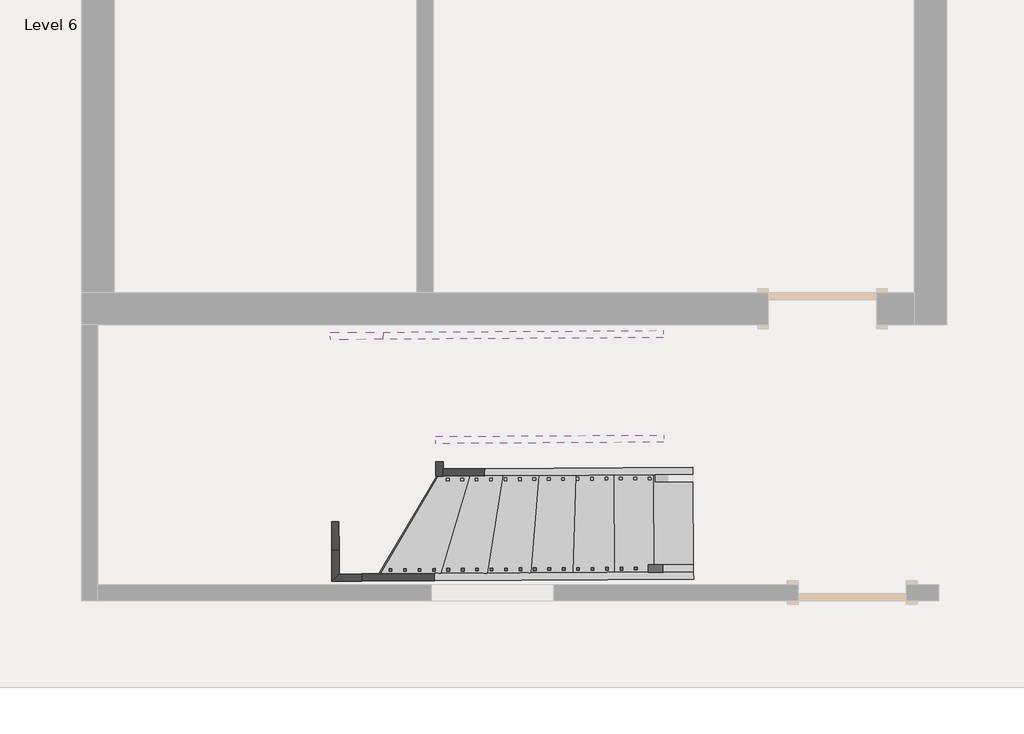
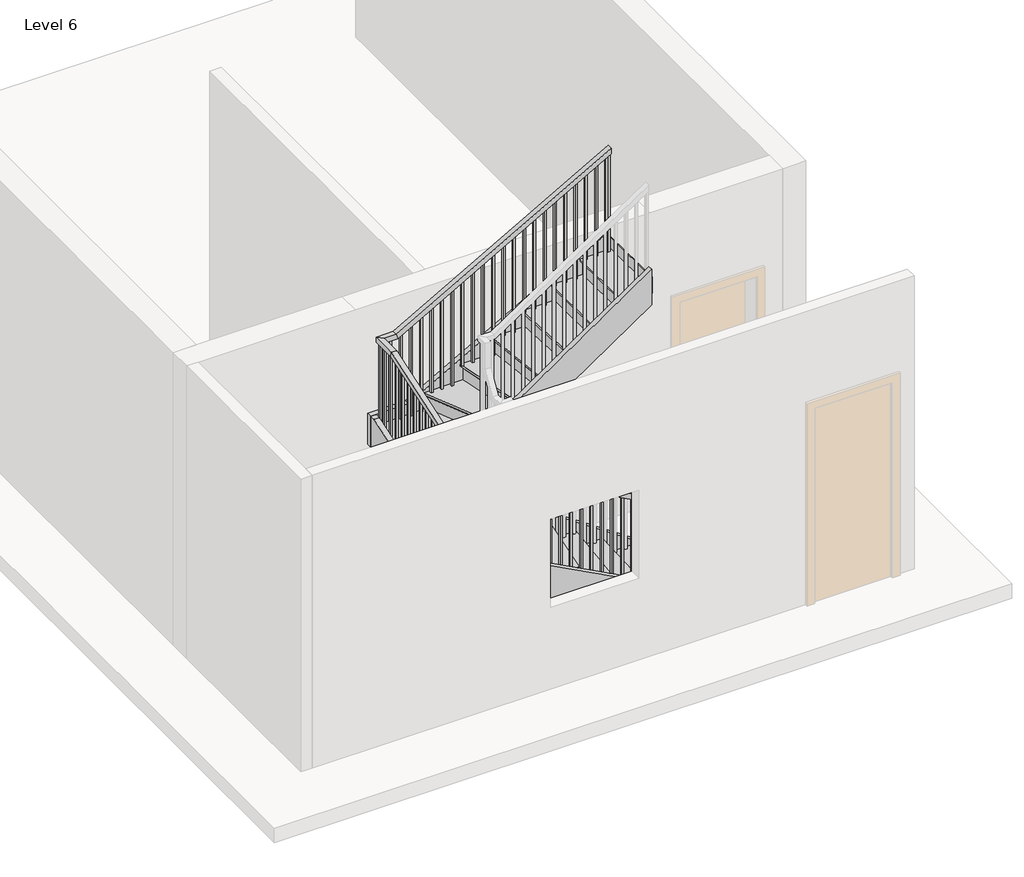
# One storey, part 2 of 2: 9 members, 1 railing, 1 stair flight.
"""IFC4 building model written with IfcOpenShell, lengths in millimetres."""

from ifc_helpers import new_model, si_unit, frame, origin, place, context, project, spatial, polyline, outline, extrude, faceted_brep, transform, mapped, element, save
from components import stair_flight_c1b2dc12

model = new_model("IFC4")

# Units and contexts
model_context = context("Model", 3, world=origin())
ifc_project = project(units=[si_unit("LENGTHUNIT", "METRE", prefix="MILLI")], contexts=[model_context])

# Site, building, storey
site = spatial("IfcSite", under=ifc_project)
building = spatial("IfcBuilding", under=site)
storey = spatial("IfcBuildingStorey", under=building, Name="Level 6", Elevation=12801.6)

# Members
placement = place(None, origin())
element("IfcMember", 1, ObjectType="Stringer - 2\" Width", at=placement, inside=storey, context=model_context, shape_type="SweptSolid", body=[
    extrude(outline(polyline([(-106.4787477, -199.0602913), (0.0, 0.0), (2650.4216713, 0.0), (2487.3820108, -304.8), (91.199922, -304.8), (-106.4787477, -199.0602913)])), frame((-116.1777511, -4276.2080688, 13027.3492487), z_axis=(-0.006129891180436152, 0.9999812120405644, 0.0), x_axis=(-0.881759529662862, -0.005405191516664865, 0.4716682263555568)), (0.0, 0.0, 1.0), 50.8),
])
element("IfcMember", 2, ObjectType="Stringer - 2\" Width", at=placement, inside=storey, context=model_context, shape_type="SweptSolid", body=[
    extrude(outline(polyline([(-2453.5237158, -4239.7350599), (-2453.2123174, -4290.5341055), (-2663.1420684, -4291.8209762), (-2612.6544213, -4240.7105322), (-2453.5237158, -4239.7350599)])), frame((0.0, 0.0, 13931.8029558), z_axis=(0.0, 0.0, 1.0), x_axis=(1.0, 0.0, 0.0)), (0.0, 0.0, 1.0), 345.6659817),
])
element("IfcMember", 3, ObjectType="Stringer - 2\" Width", at=placement, inside=storey, context=model_context, shape_type="SweptSolid", body=[
    extrude(outline(polyline([(-2612.6544213, -4240.7105322), (-2663.1420684, -4291.8209762), (-2664.4731567, -4074.6779247), (-2613.6741111, -4074.3665263), (-2612.6544213, -4240.7105322)])), frame((0.0, 0.0, 13931.8029558), z_axis=(0.0, 0.0, 1.0), x_axis=(1.0, 0.0, 0.0)), (0.0, 0.0, 1.0), 345.6659817),
])
element("IfcMember", 4, ObjectType="Stringer - 2\" Width", at=placement, inside=storey, context=model_context, shape_type="SweptSolid", body=[
    extrude(outline(polyline([(-112.9595567, -326.688092), (0.0, 0.0), (1516.7940002, 1e-07), (1565.1210838, -16.7101466), (1457.9394259, -326.6880919), (-112.9595567, -326.688092)])), frame((-2664.4731567, -4074.6779247, 14277.4689375), z_axis=(0.9999812120405643, 0.006129891180436421, 0.0), x_axis=(-0.005793345483301546, 0.9450798501367781, 0.3267881791215163)), (0.0, 0.0, 1.0), 50.8),
])
element("IfcMember", 5, ObjectType="Stringer - 2\" Width", at=placement, inside=storey, context=model_context, shape_type="SweptSolid", body=[
    extrude(outline(polyline([(-111.800968, -163.7049666), (0.0, 0.0), (2130.8093531, 0.0), (1922.648686, -304.8000001), (94.7979387, -304.8000001), (-111.800968, -163.7049666)])), frame((-120.6930289, -3539.621908, 12999.8391801), z_axis=(-0.006129891180436334, 0.9999812120405643, 0.0), x_axis=(-0.8257797012408892, -0.005062034812924604, 0.5639700885880922)), (0.0, 0.0, 1.0), 50.8),
])
element("IfcMember", 6, ObjectType="Stringer - 2\" Width", at=placement, inside=storey, context=model_context, shape_type="SweptSolid", body=[
    extrude(outline(polyline([(-476.3090819, -288.3824073), (0.0, 0.0), (441.380003, 0.0), (-62.0453256, -304.8), (-466.3690133, -304.8), (-476.3090819, -288.3824073)])), frame((-1931.0711854, -3550.7195376, 14423.9542381), z_axis=(0.9999812120405644, 0.006129891180436035, 0.0), x_axis=(-0.0031747997513555445, 0.5179113315223277, 0.8554284150806007)), (0.0, 0.0, 1.0), 50.8),
])
element("IfcMember", 7, ObjectType="Stringer - 2\" Width", at=placement, inside=storey, context=model_context, shape_type="SweptSolid", body=[
    extrude(outline(polyline([(205.0123517, -304.8), (0.0, 0.0), (1938.1040339, 0.0), (2143.1163855, -304.8), (205.0123517, -304.8)])), frame((-1932.4724786, -3322.1238325, 14468.5006308), z_axis=(-0.006129891180436482, 0.9999812120405644, 0.0), x_axis=(0.8297505463599371, 0.005086376118722323, 0.5581112430271987)), (0.0, 0.0, 1.0), 50.8),
])
element("IfcMember", 8, ObjectType="Stringer - 2\" Width", at=placement, inside=storey, context=model_context, shape_type="SweptSolid", body=[
    extrude(outline(polyline([(-2673.5739172, -2590.0529496), (-2673.8853157, -2539.253904), (-2303.2697085, -2536.982028), (-2302.9583101, -2587.7810735), (-2673.5739172, -2590.0529496)])), frame((0.0, 0.0, 14450.6329153), z_axis=(0.0, 0.0, 1.0), x_axis=(1.0, 0.0, 0.0)), (0.0, 0.0, 1.0), 322.5063717),
])
element("IfcMember", 9, ObjectType="Stringer - 2\" Width", at=placement, inside=storey, context=model_context, shape_type="SweptSolid", body=[
    extrude(outline(polyline([(155.3220552, -282.6400873), (0.0, 0.0), (2252.6037587, 1e-07), (2407.9258139, -282.6400872), (155.3220552, -282.6400873)])), frame((-2302.9583101, -2587.7810735, 14450.6329153), z_axis=(-0.006129891180436272, 0.9999812120405644, 0.0), x_axis=(0.8763695910030255, 0.005372151158450034, 0.4816092606637882)), (0.0, 0.0, 1.0), 50.8),
])

# Railing
element("IfcRailing", 10, ObjectType="Handrail - Rectangular", at=placement, inside=storey, context=model_context, shape_type="SolidModel", body=[
    faceted_brep([(-116.4891496, -4225.4090232, 13885.3333333), (-116.4891496, -4225.4090232, 13827.5022634), (-116.800548, -4174.6099776, 13827.5022634), (-116.800548, -4174.6099776, 13885.3333333), (-2474.2717021, -4239.8622452, 15168.0653479), (-2487.1954725, -4239.941468, 15117.2653479), (-2487.506871, -4189.1424224, 15117.2653479), (-2474.5831006, -4189.0631997, 15168.0653479), (-2612.6544213, -4240.7105322, 15168.0653479), (-2612.6544213, -4240.7105322, 15117.2653479), (-2562.1667742, -4189.6000881, 15117.2653479), (-2562.1667742, -4189.6000881, 15168.0653479), (-2613.899826, -4037.5452114, 15168.0653479), (-2613.9521428, -4029.010664, 15117.2653479), (-2563.1530973, -4028.6992655, 15117.2653479), (-2563.1007804, -4037.2338129, 15168.0653479), (-2621.180916, -2849.7666717, 15578.7734867), (-2621.2332328, -2841.2321243, 15527.9734867), (-2570.4341872, -2840.9207258, 15527.9734867), (-2570.3818704, -2849.4552732, 15578.7734867), (-2622.7748716, -2589.7415511, 15578.7734867), (-2622.7748716, -2589.7415511, 15527.9734867), (-2571.6644276, -2640.2291982, 15527.9734867), (-2571.6644276, -2640.2291982, 15578.7734867), (-2452.0429693, -2588.6949634, 15578.7734867), (-2438.8245474, -2588.6139344, 15527.9734867), (-2438.513149, -2639.41298, 15527.9734867), (-2451.7315708, -2639.494009, 15578.7734867), (-328.8448754, -2575.6797456, 16764.0), (-328.533477, -2626.4787912, 16764.0), (-328.533477, -2626.4787912, 16705.82112), (-328.8448754, -2575.6797456, 16705.82112)], [[[0, 1, 2, 3]], [[1, 0, 4, 5]], [[2, 1, 5, 6]], [[3, 2, 6, 7]], [[0, 3, 7, 4]], [[5, 4, 8, 9]], [[6, 5, 9, 10]], [[7, 6, 10, 11]], [[4, 7, 11, 8]], [[9, 8, 12, 13]], [[10, 9, 13, 14]], [[11, 10, 14, 15]], [[8, 11, 15, 12]], [[13, 12, 16, 17]], [[14, 13, 17, 18]], [[15, 14, 18, 19]], [[12, 15, 19, 16]], [[17, 16, 20, 21]], [[18, 17, 21, 22]], [[19, 18, 22, 23]], [[16, 19, 23, 20]], [[21, 20, 24, 25]], [[22, 21, 25, 26]], [[23, 22, 26, 27]], [[20, 23, 27, 24]], [[28, 29, 30, 31]], [[25, 24, 28, 31]], [[26, 25, 31, 30]], [[27, 26, 30, 29]], [[24, 27, 29, 28]]]),
    extrude(outline(polyline([(233.9170124, 19.05), (1235.5250403, 19.05), (1235.5250403, 0.0), (223.2829877, 0.0), (233.9170124, 19.05)])), frame((-352.4784362, -2610.7502757, 16915.791707), z_axis=(-0.0061298911804362555, 0.9999812120405644, 0.0), x_axis=(0.0, 0.0, -1.0)), (0.0, 0.0, 1.0), 19.05),
    extrude(outline(polyline([(233.9170123, 19.05), (1178.8102421, 19.05), (1178.8102421, 0.0), (223.2829877, 0.0), (233.9170123, 19.05)])), frame((-454.0765273, -2611.3730726, 16859.0769088), z_axis=(-0.0061298911804362555, 0.9999812120405644, 0.0), x_axis=(0.0, 0.0, -1.0)), (0.0, 0.0, 1.0), 19.05),
    extrude(outline(polyline([(233.9170124, 19.05), (1122.095444, 19.05), (1122.095444, 0.0), (223.2829877, 0.0), (233.9170124, 19.05)])), frame((-555.6746185, -2611.9958696, 16802.3621107), z_axis=(-0.0061298911804362555, 0.9999812120405644, 0.0), x_axis=(0.0, 0.0, -1.0)), (0.0, 0.0, 1.0), 19.05),
    extrude(outline(polyline([(233.9170123, 19.05), (1234.7139792, 19.05), (1234.7139792, 0.0), (223.2829877, 0.0), (233.9170123, 19.05)])), frame((-657.2727096, -2612.6186665, 16745.6473125), z_axis=(-0.0061298911804362555, 0.9999812120405644, 0.0), x_axis=(0.0, 0.0, -1.0)), (0.0, 0.0, 1.0), 19.05),
    extrude(outline(polyline([(233.9170123, 19.05), (1177.999181, 19.05), (1177.999181, 0.0), (223.2829876, 0.0), (233.9170123, 19.05)])), frame((-758.8708008, -2613.2414635, 16688.9325143), z_axis=(-0.0061298911804362555, 0.9999812120405644, 0.0), x_axis=(0.0, 0.0, -1.0)), (0.0, 0.0, 1.0), 19.05),
    extrude(outline(polyline([(233.9170123, 19.05), (1121.2843829, 19.05), (1121.2843829, 0.0), (223.2829877, 0.0), (233.9170123, 19.05)])), frame((-860.4688919, -2613.8642604, 16632.2177162), z_axis=(-0.0061298911804362555, 0.9999812120405644, 0.0), x_axis=(0.0, 0.0, -1.0)), (0.0, 0.0, 1.0), 19.05),
    extrude(outline(polyline([(233.9170123, 19.0499999), (1233.902918, 19.0499999), (1233.902918, 0.0), (223.2829876, 0.0), (233.9170123, 19.0499999)])), frame((-962.0669831, -2614.4870574, 16575.502918), z_axis=(-0.0061298911804362555, 0.9999812120405644, 0.0), x_axis=(0.0, 0.0, -1.0)), (0.0, 0.0, 1.0), 19.05),
    extrude(outline(polyline([(233.9170123, 19.05), (1177.1881199, 19.05), (1177.1881199, 0.0), (223.2829877, 0.0), (233.9170123, 19.05)])), frame((-1063.6650742, -2615.1098543, 16518.7881199), z_axis=(-0.0061298911804362555, 0.9999812120405644, 0.0), x_axis=(0.0, 0.0, -1.0)), (0.0, 0.0, 1.0), 19.05),
    extrude(outline(polyline([(233.9170123, 19.05), (1120.4733217, 19.05), (1120.4733217, 0.0), (223.2829876, 0.0), (233.9170123, 19.05)])), frame((-1165.2631653, -2615.7326513, 16462.0733217), z_axis=(-0.0061298911804362555, 0.9999812120405644, 0.0), x_axis=(0.0, 0.0, -1.0)), (0.0, 0.0, 1.0), 19.05),
    extrude(outline(polyline([(233.9170123, 19.05), (1233.0918569, 19.05), (1233.0918569, 0.0), (223.2829877, 0.0), (233.9170123, 19.05)])), frame((-1266.8612565, -2616.3554482, 16405.3585236), z_axis=(-0.0061298911804362555, 0.9999812120405644, 0.0), x_axis=(0.0, 0.0, -1.0)), (0.0, 0.0, 1.0), 19.05),
    extrude(outline(polyline([(233.9170123, 19.05), (1176.3770587, 19.05), (1176.3770587, 0.0), (223.2829876, 0.0), (233.9170123, 19.05)])), frame((-1368.4593476, -2616.9782451, 16348.6437254), z_axis=(-0.0061298911804362555, 0.9999812120405644, 0.0), x_axis=(0.0, 0.0, -1.0)), (0.0, 0.0, 1.0), 19.05),
    extrude(outline(polyline([(233.9170123, 19.05), (1288.995594, 19.05), (1288.995594, 0.0), (223.2829877, 0.0), (233.9170123, 19.05)])), frame((-1470.0574388, -2617.6010421, 16291.9289273), z_axis=(-0.0061298911804362555, 0.9999812120405644, 0.0), x_axis=(0.0, 0.0, -1.0)), (0.0, 0.0, 1.0), 19.05),
    extrude(outline(polyline([(233.9170123, 19.05), (1232.2807958, 19.05), (1232.2807958, 0.0), (223.2829876, 0.0), (233.9170123, 19.05)])), frame((-1571.6555299, -2618.223839, 16235.2141291), z_axis=(-0.0061298911804362555, 0.9999812120405644, 0.0), x_axis=(0.0, 0.0, -1.0)), (0.0, 0.0, 1.0), 19.05),
    extrude(outline(polyline([(233.9170123, 19.05), (1175.5659977, 19.05), (1175.5659977, 0.0), (223.2829877, 0.0), (233.9170123, 19.05)])), frame((-1673.2536211, -2618.846636, 16178.499331), z_axis=(-0.0061298911804362555, 0.9999812120405644, 0.0), x_axis=(0.0, 0.0, -1.0)), (0.0, 0.0, 1.0), 19.05),
    extrude(outline(polyline([(233.9170123, 19.05), (1118.8511995, 19.05), (1118.8511995, 0.0), (223.2829876, 0.0), (233.9170123, 19.05)])), frame((-1774.8517122, -2619.4694329, 16121.7845328), z_axis=(-0.0061298911804362555, 0.9999812120405644, 0.0), x_axis=(0.0, 0.0, -1.0)), (0.0, 0.0, 1.0), 19.05),
    extrude(outline(polyline([(233.9170123, 19.05), (1231.4697347, 19.05), (1231.4697347, 0.0), (223.2829877, 0.0), (233.9170123, 19.05)])), frame((-1876.4498033, -2620.0922299, 16065.0697347), z_axis=(-0.0061298911804362555, 0.9999812120405644, 0.0), x_axis=(0.0, 0.0, -1.0)), (0.0, 0.0, 1.0), 19.05),
    extrude(outline(polyline([(233.9170123, 19.05), (1174.7549365, 19.05), (1174.7549365, 0.0), (223.2829876, 0.0), (233.9170123, 19.05)])), frame((-1978.0478945, -2620.7150268, 16008.3549365), z_axis=(-0.0061298911804362555, 0.9999812120405644, 0.0), x_axis=(0.0, 0.0, -1.0)), (0.0, 0.0, 1.0), 19.05),
    extrude(outline(polyline([(233.9170124, 19.05), (1118.0401384, 19.05), (1118.0401384, 0.0), (223.2829877, 0.0), (233.9170124, 19.05)])), frame((-2079.6459856, -2621.3378238, 15951.6401384), z_axis=(-0.0061298911804362555, 0.9999812120405644, 0.0), x_axis=(0.0, 0.0, -1.0)), (0.0, 0.0, 1.0), 19.05),
    extrude(outline(polyline([(233.9170123, 19.05), (1230.6586735, 19.05), (1230.6586735, 0.0), (223.2829876, 0.0), (233.9170123, 19.05)])), frame((-2181.2440768, -2621.9606207, 15894.9253402), z_axis=(-0.0061298911804362555, 0.9999812120405644, 0.0), x_axis=(0.0, 0.0, -1.0)), (0.0, 0.0, 1.0), 19.05),
    extrude(outline(polyline([(233.9170124, 19.05), (1173.9438754, 19.05), (1173.9438754, 0.0), (223.2829877, 0.0), (233.9170124, 19.05)])), frame((-2282.8421679, -2622.5834176, 15838.2105421), z_axis=(-0.0061298911804362555, 0.9999812120405644, 0.0), x_axis=(0.0, 0.0, -1.0)), (0.0, 0.0, 1.0), 19.05),
    extrude(outline(polyline([(233.9170123, 19.05), (1117.2290772, 19.05), (1117.2290772, 0.0), (223.2829877, 0.0), (233.9170123, 19.05)])), frame((-2384.4402591, -2623.2062146, 15781.4957439), z_axis=(-0.0061298911804362555, 0.9999812120405644, 0.0), x_axis=(0.0, 0.0, -1.0)), (0.0, 0.0, 1.0), 19.05),
    extrude(outline(polyline([(-2505.2047667, -2604.8961439), (-2486.1551246, -2604.7793694), (-2486.0383502, -2623.8290115), (-2505.0879923, -2623.945786), (-2505.2047667, -2604.8961439)])), frame((0.0, 0.0, 14664.2666667), z_axis=(0.0, 0.0, 1.0), x_axis=(1.0, 0.0, 0.0)), (0.0, 0.0, 1.0), 863.70682),
    extrude(outline(polyline([(-2606.2189857, -2700.7671513), (-2606.3357602, -2681.7175092), (-2587.2861181, -2681.6007347), (-2587.1693436, -2700.6503768), (-2606.2189857, -2700.7671513)])), frame((0.0, 0.0, 14664.2666667), z_axis=(0.0, 0.0, 1.0), x_axis=(1.0, 0.0, 0.0)), (0.0, 0.0, 1.0), 863.70682),
    extrude(outline(polyline([(-2605.5961888, -2802.3652424), (-2605.7129632, -2783.3156003), (-2586.6633211, -2783.1988259), (-2586.5465467, -2802.248468), (-2605.5961888, -2802.3652424)])), frame((0.0, 0.0, 14664.2666667), z_axis=(0.0, 0.0, 1.0), x_axis=(1.0, 0.0, 0.0)), (0.0, 0.0, 1.0), 863.70682),
    extrude(outline(polyline([(225.3065228, 19.0499999), (1243.2088863, 19.0499999), (1243.2088863, 0.0), (231.8934772, 0.0), (225.3065228, 19.0499999)])), frame((-2604.9733918, -2903.9633335, 15738.1422196), z_axis=(0.9999812120405643, 0.0061298911804362685, 0.0), x_axis=(0.0, 0.0, -1.0)), (0.0, 0.0, 1.0), 19.05),
    extrude(outline(polyline([(225.3065229, 19.05), (1208.078463, 19.05), (1208.078463, 0.0), (231.8934772, 0.0), (225.3065229, 19.05)])), frame((-2604.3505949, -3005.5614247, 15703.0117963), z_axis=(0.9999812120405643, 0.0061298911804362685, 0.0), x_axis=(0.0, 0.0, -1.0)), (0.0, 0.0, 1.0), 19.05),
    extrude(outline(polyline([(225.3065228, 19.05), (1172.9480396, 19.05), (1172.9480396, 0.0), (231.8934772, 0.0), (225.3065228, 19.05)])), frame((-2603.727798, -3107.1595158, 15667.8813729), z_axis=(0.9999812120405643, 0.0061298911804362685, 0.0), x_axis=(0.0, 0.0, -1.0)), (0.0, 0.0, 1.0), 19.05),
    extrude(outline(polyline([(225.3065228, 19.05), (1137.8176163, 19.05), (1137.8176163, 0.0), (231.8934772, 0.0), (225.3065228, 19.05)])), frame((-2603.105001, -3208.757607, 15632.7509496), z_axis=(0.9999812120405643, 0.0061298911804362685, 0.0), x_axis=(0.0, 0.0, -1.0)), (0.0, 0.0, 1.0), 19.05),
    extrude(outline(polyline([(225.3065228, 19.05), (1102.687193, 19.05), (1102.687193, 0.0), (231.8934772, 0.0), (225.3065228, 19.05)])), frame((-2602.4822041, -3310.3556981, 15597.6205263), z_axis=(0.9999812120405643, 0.0061298911804362685, 0.0), x_axis=(0.0, 0.0, -1.0)), (0.0, 0.0, 1.0), 19.05),
    extrude(outline(polyline([(225.3065228, 19.05), (1236.890103, 19.05), (1236.890103, 0.0), (231.8934772, 0.0), (225.3065228, 19.05)])), frame((-2601.8594071, -3411.9537893, 15562.490103), z_axis=(0.9999812120405643, 0.0061298911804362685, 0.0), x_axis=(0.0, 0.0, -1.0)), (0.0, 0.0, 1.0), 19.05),
    extrude(outline(polyline([(225.3065229, 19.05), (1201.7596797, 19.05), (1201.7596797, 0.0), (231.8934772, 0.0), (225.3065229, 19.05)])), frame((-2601.2366102, -3513.5518804, 15527.3596797), z_axis=(0.9999812120405643, 0.0061298911804362685, 0.0), x_axis=(0.0, 0.0, -1.0)), (0.0, 0.0, 1.0), 19.05),
    extrude(outline(polyline([(225.3065228, 19.0499999), (1166.6292563, 19.0499999), (1166.6292563, 0.0), (231.8934772, 0.0), (225.3065228, 19.0499999)])), frame((-2600.6138132, -3615.1499715, 15492.2292563), z_axis=(0.9999812120405643, 0.0061298911804362685, 0.0), x_axis=(0.0, 0.0, -1.0)), (0.0, 0.0, 1.0), 19.05),
    extrude(outline(polyline([(225.3065228, 19.05), (1131.498833, 19.05), (1131.498833, 0.0), (231.8934772, 0.0), (225.3065228, 19.05)])), frame((-2599.9910163, -3716.7480627, 15457.098833), z_axis=(0.9999812120405643, 0.0061298911804362685, 0.0), x_axis=(0.0, 0.0, -1.0)), (0.0, 0.0, 1.0), 19.05),
    extrude(outline(polyline([(225.3065228, 19.05), (1096.3684097, 19.05), (1096.3684097, 0.0), (231.8934772, 0.0), (225.3065228, 19.05)])), frame((-2599.3682194, -3818.3461538, 15421.9684097), z_axis=(0.9999812120405643, 0.0061298911804362685, 0.0), x_axis=(0.0, 0.0, -1.0)), (0.0, 0.0, 1.0), 19.05),
    extrude(outline(polyline([(225.3065228, 19.05), (1230.5713197, 19.05), (1230.5713197, 0.0), (231.8934772, 0.0), (225.3065228, 19.05)])), frame((-2598.7454224, -3919.944245, 15386.8379864), z_axis=(0.9999812120405643, 0.0061298911804362685, 0.0), x_axis=(0.0, 0.0, -1.0)), (0.0, 0.0, 1.0), 19.05),
    extrude(outline(polyline([(225.3065228, 19.05), (1195.4408963, 19.05), (1195.4408963, 0.0), (231.8934771, 0.0), (225.3065228, 19.05)])), frame((-2598.1226255, -4021.5423361, 15351.707563), z_axis=(0.9999812120405643, 0.0061298911804362685, 0.0), x_axis=(0.0, 0.0, -1.0)), (0.0, 0.0, 1.0), 19.05),
    extrude(outline(polyline([(-2597.4998285, -4123.1404273), (-2597.6166029, -4104.0907852), (-2578.5669609, -4103.9740107), (-2578.4501864, -4123.0236528), (-2597.4998285, -4123.1404273)])), frame((0.0, 0.0, 14156.2666667), z_axis=(0.0, 0.0, 1.0), x_axis=(1.0, 0.0, 0.0)), (0.0, 0.0, 1.0), 960.9986813),
    extrude(outline(polyline([(-2545.415828, -4224.4230609), (-2564.4654701, -4224.5398353), (-2564.5822445, -4205.4901932), (-2545.5326024, -4205.3734188), (-2545.415828, -4224.4230609)])), frame((0.0, 0.0, 14156.2666667), z_axis=(0.0, 0.0, 1.0), x_axis=(1.0, 0.0, 0.0)), (0.0, 0.0, 1.0), 960.9986813),
    extrude(outline(polyline([(223.4181002, 19.05), (1171.1283424, 19.05), (1171.1283424, 0.0), (233.7818998, 0.0), (223.4181002, 19.05)])), frame((-2443.8177368, -4223.800264, 15327.3950091), z_axis=(-0.006129891180436165, 0.9999812120405643, 0.0), x_axis=(0.0, 0.0, -1.0)), (0.0, 0.0, 1.0), 19.05),
    extrude(outline(polyline([(223.4181002, 19.05), (1115.8547448, 19.05), (1115.8547448, 0.0), (233.7818998, 0.0), (223.4181002, 19.05)])), frame((-2342.2196457, -4223.177467, 15272.1214115), z_axis=(-0.006129891180436165, 0.9999812120405643, 0.0), x_axis=(0.0, 0.0, -1.0)), (0.0, 0.0, 1.0), 19.05),
    extrude(outline(polyline([(223.4181002, 19.05), (1229.9144805, 19.05), (1229.9144805, 0.0), (233.7818997, 0.0), (223.4181002, 19.05)])), frame((-2240.6215545, -4222.5546701, 15216.8478138), z_axis=(-0.006129891180436165, 0.9999812120405643, 0.0), x_axis=(0.0, 0.0, -1.0)), (0.0, 0.0, 1.0), 19.05),
    extrude(outline(polyline([(223.4181002, 19.05), (1174.6408829, 19.05), (1174.6408829, 0.0), (233.7818998, 0.0), (223.4181002, 19.05)])), frame((-2139.0234634, -4221.9318731, 15161.5742162), z_axis=(-0.006129891180436165, 0.9999812120405643, 0.0), x_axis=(0.0, 0.0, -1.0)), (0.0, 0.0, 1.0), 19.05),
    extrude(outline(polyline([(223.4181003, 19.0499999), (1119.3672853, 19.0499999), (1119.3672853, 0.0), (233.7818998, 0.0), (223.4181003, 19.0499999)])), frame((-2037.4253723, -4221.3090762, 15106.3006186), z_axis=(-0.006129891180436165, 0.9999812120405643, 0.0), x_axis=(0.0, 0.0, -1.0)), (0.0, 0.0, 1.0), 19.05),
    extrude(outline(polyline([(223.4181002, 19.05), (1064.0936876, 19.05), (1064.0936876, 0.0), (233.7818998, 0.0), (223.4181002, 19.05)])), frame((-1935.8272811, -4220.6862792, 15051.0270209), z_axis=(-0.006129891180436165, 0.9999812120405643, 0.0), x_axis=(0.0, 0.0, -1.0)), (0.0, 0.0, 1.0), 19.05),
    extrude(outline(polyline([(223.4181002, 19.05), (1178.1534233, 19.05), (1178.1534233, 0.0), (233.7818998, 0.0), (223.4181002, 19.05)])), frame((-1834.22919, -4220.0634823, 14995.7534233), z_axis=(-0.006129891180436165, 0.9999812120405643, 0.0), x_axis=(0.0, 0.0, -1.0)), (0.0, 0.0, 1.0), 19.05),
    extrude(outline(polyline([(223.4181002, 19.05), (1122.8798256, 19.05), (1122.8798256, 0.0), (233.7818997, 0.0), (223.4181002, 19.05)])), frame((-1732.6310988, -4219.4406854, 14940.4798256), z_axis=(-0.006129891180436165, 0.9999812120405643, 0.0), x_axis=(0.0, 0.0, -1.0)), (0.0, 0.0, 1.0), 19.05),
    extrude(outline(polyline([(223.4181002, 19.05), (1067.606228, 19.05), (1067.606228, 0.0), (233.7818998, 0.0), (223.4181002, 19.05)])), frame((-1631.0330077, -4218.8178884, 14885.206228), z_axis=(-0.006129891180436165, 0.9999812120405643, 0.0), x_axis=(0.0, 0.0, -1.0)), (0.0, 0.0, 1.0), 19.05),
    extrude(outline(polyline([(223.4181003, 19.05), (1181.6659637, 19.05), (1181.6659637, 0.0), (233.7818998, 0.0), (223.4181003, 19.05)])), frame((-1529.4349165, -4218.1950915, 14829.9326304), z_axis=(-0.006129891180436165, 0.9999812120405643, 0.0), x_axis=(0.0, 0.0, -1.0)), (0.0, 0.0, 1.0), 19.05),
    extrude(outline(polyline([(223.4181002, 19.05), (1126.392366, 19.05), (1126.392366, 0.0), (233.7818998, 0.0), (223.4181002, 19.05)])), frame((-1427.8368254, -4217.5722945, 14774.6590327), z_axis=(-0.006129891180436165, 0.9999812120405643, 0.0), x_axis=(0.0, 0.0, -1.0)), (0.0, 0.0, 1.0), 19.05),
    extrude(outline(polyline([(223.4181002, 19.0499999), (1071.1187684, 19.0499999), (1071.1187684, 0.0), (233.7818998, 0.0), (223.4181002, 19.0499999)])), frame((-1326.2387343, -4216.9494976, 14719.3854351), z_axis=(-0.006129891180436165, 0.9999812120405643, 0.0), x_axis=(0.0, 0.0, -1.0)), (0.0, 0.0, 1.0), 19.05),
    extrude(outline(polyline([(223.4181002, 19.05), (1185.1785041, 19.05), (1185.1785041, 0.0), (233.7818997, 0.0), (223.4181002, 19.05)])), frame((-1224.6406431, -4216.3267006, 14664.1118374), z_axis=(-0.006129891180436165, 0.9999812120405643, 0.0), x_axis=(0.0, 0.0, -1.0)), (0.0, 0.0, 1.0), 19.05),
    extrude(outline(polyline([(223.4181002, 19.05), (1129.9049065, 19.05), (1129.9049065, 0.0), (233.7818998, 0.0), (223.4181002, 19.05)])), frame((-1123.042552, -4215.7039037, 14608.8382398), z_axis=(-0.006129891180436165, 0.9999812120405643, 0.0), x_axis=(0.0, 0.0, -1.0)), (0.0, 0.0, 1.0), 19.05),
    extrude(outline(polyline([(223.4181003, 19.05), (1074.6313089, 19.05), (1074.6313089, 0.0), (233.7818998, 0.0), (223.4181003, 19.05)])), frame((-1021.4444608, -4215.0811067, 14553.5646422), z_axis=(-0.006129891180436165, 0.9999812120405643, 0.0), x_axis=(0.0, 0.0, -1.0)), (0.0, 0.0, 1.0), 19.05),
    extrude(outline(polyline([(223.4181002, 19.05), (1188.6910445, 19.05), (1188.6910445, 0.0), (233.7818998, 0.0), (223.4181002, 19.05)])), frame((-919.8463697, -4214.4583098, 14498.2910445), z_axis=(-0.006129891180436165, 0.9999812120405643, 0.0), x_axis=(0.0, 0.0, -1.0)), (0.0, 0.0, 1.0), 19.05),
    extrude(outline(polyline([(223.4181002, 19.05), (1133.4174469, 19.05), (1133.4174469, 0.0), (233.7818998, 0.0), (223.4181002, 19.05)])), frame((-818.2482785, -4213.8355129, 14443.0174469), z_axis=(-0.006129891180436165, 0.9999812120405643, 0.0), x_axis=(0.0, 0.0, -1.0)), (0.0, 0.0, 1.0), 19.05),
    extrude(outline(polyline([(223.4181002, 19.05), (1078.1438492, 19.05), (1078.1438492, 0.0), (233.7818997, 0.0), (223.4181002, 19.05)])), frame((-716.6501874, -4213.2127159, 14387.7438492), z_axis=(-0.006129891180436165, 0.9999812120405643, 0.0), x_axis=(0.0, 0.0, -1.0)), (0.0, 0.0, 1.0), 19.05),
    extrude(outline(polyline([(223.4181002, 19.0499999), (1192.2035849, 19.0499999), (1192.2035849, 0.0), (233.7818998, 0.0), (223.4181002, 19.0499999)])), frame((-615.0520963, -4212.589919, 14332.4702516), z_axis=(-0.006129891180436165, 0.9999812120405643, 0.0), x_axis=(0.0, 0.0, -1.0)), (0.0, 0.0, 1.0), 19.05),
    extrude(outline(polyline([(223.4181003, 19.05), (1136.9299873, 19.05), (1136.9299873, 0.0), (233.7818998, 0.0), (223.4181003, 19.05)])), frame((-513.4540051, -4211.967122, 14277.196654), z_axis=(-0.006129891180436165, 0.9999812120405643, 0.0), x_axis=(0.0, 0.0, -1.0)), (0.0, 0.0, 1.0), 19.05),
    extrude(outline(polyline([(223.4181002, 19.05), (1081.6563896, 19.05), (1081.6563896, 0.0), (233.7818998, 0.0), (223.4181002, 19.05)])), frame((-411.855914, -4211.3443251, 14221.9230563), z_axis=(-0.006129891180436165, 0.9999812120405643, 0.0), x_axis=(0.0, 0.0, -1.0)), (0.0, 0.0, 1.0), 19.05),
    extrude(outline(polyline([(223.4181002, 19.05), (1195.7161254, 19.05), (1195.7161254, 0.0), (233.7818998, 0.0), (223.4181002, 19.05)])), frame((-310.2578228, -4210.7215281, 14166.6494587), z_axis=(-0.006129891180436165, 0.9999812120405643, 0.0), x_axis=(0.0, 0.0, -1.0)), (0.0, 0.0, 1.0), 19.05),
    extrude(outline(polyline([(223.4181002, 19.05), (1140.4425277, 19.05), (1140.4425277, 0.0), (233.7818997, 0.0), (223.4181002, 19.05)])), frame((-208.6597317, -4210.0987312, 14111.375861), z_axis=(-0.006129891180436165, 0.9999812120405643, 0.0), x_axis=(0.0, 0.0, -1.0)), (0.0, 0.0, 1.0), 19.05),
    extrude(outline(polyline([(-2606.6860834, -2624.5685829), (-2606.8028579, -2605.5189408), (-2587.7532158, -2605.4021664), (-2587.6364414, -2624.4518085), (-2606.6860834, -2624.5685829)])), frame((0.0, 0.0, 14664.2666667), z_axis=(0.0, 0.0, 1.0), x_axis=(1.0, 0.0, 0.0)), (0.0, 0.0, 1.0), 863.70682),
    extrude(outline(polyline([(-2577.8273895, -4224.621744), (-2596.8770316, -4224.7385184), (-2596.993806, -4205.6888763), (-2577.9441639, -4205.5721019), (-2577.8273895, -4224.621744)])), frame((0.0, 0.0, 14156.2666667), z_axis=(0.0, 0.0, 1.0), x_axis=(1.0, 0.0, 0.0)), (0.0, 0.0, 1.0), 960.9986813),
    extrude(outline(polyline([(233.9170123, 19.05), (1248.8374409, 19.05), (1248.8374409, 0.0), (223.2829876, 0.0), (233.9170123, 19.05)])), frame((-328.630789, -2610.6040895, 16929.1041076), z_axis=(-0.0061298911804362555, 0.9999812120405644, 0.0), x_axis=(0.0, 0.0, -1.0)), (0.0, 0.0, 1.0), 19.05),
    extrude(outline(polyline([(223.4181002, 19.05), (1090.3508299, 19.05), (1090.3508299, 0.0), (233.7818998, 0.0), (223.4181002, 19.05)])), frame((-116.5864616, -4209.5343215, 14061.2841632), z_axis=(-0.006129891180436165, 0.9999812120405643, 0.0), x_axis=(0.0, 0.0, -1.0)), (0.0, 0.0, 1.0), 19.05),
])

# Stair flight
stair_flight_shape = stair_flight_c1b2dc12(model_context)
element("IfcStairFlight", 11, ObjectType="2\" Tread 1\" Nosing 1/4\" Riser", at=placement, inside=storey, context=model_context, shape_type="MappedRepresentation", body=[
    mapped(stair_flight_shape, transform((0.0, 0.0, 0.0), x_axis=(1.0, 0.0, 0.0), y_axis=(0.0, 1.0, 0.0), z_axis=(0.0, 0.0, 1.0))),
])

save(model, "model.ifc")

# Revit data of these elements
# Type "Handrail - Rectangular"
#   Assembly Code = "C2010400"
#   built-in parameter 1008612 = 0.0416667 (stored number, unit not read)
#   built-in parameter 1008611 = 0.0416667 (stored number, unit not read)
#   built-in parameter 1008609 = 0.333333 (stored number, unit not read)
#   built-in parameter 1008604 = 0.166667 (stored number, unit not read)
#   built-in parameter 1008603 = 0.166667 (stored number, unit not read)
#   Railing Height = 3' - 0"
#   built-in parameter 1008630 = 2
#   built-in parameter 1008610 = 2
#   built-in parameter 1008618 = Baluster - Square : 3/4"
# Elements 1, 2, 3, 4, 5, 6, 7, 8, 9 (IfcMember, "Stringer - 2\" Width")
#   Phase Created = New Construction
# Element 10 (IfcRailing, "Handrail - Rectangular")
#   Phase Created = New Construction
# Element 11 (IfcStairFlight, "2\" Tread 1\" Nosing 1/4\" Riser")
#   Phase Created = New Construction
